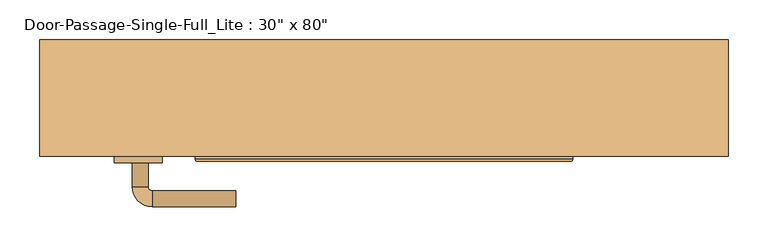
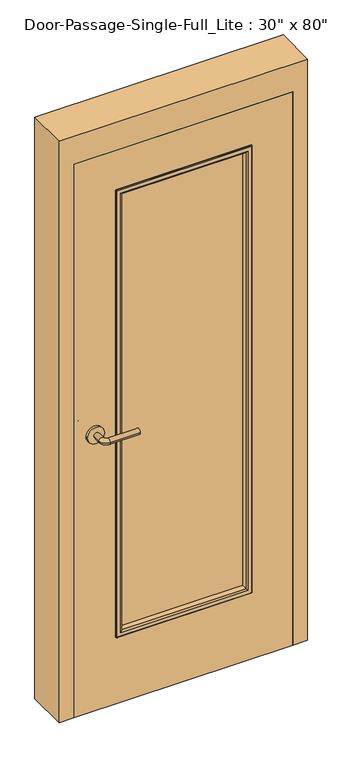
"""IFC4 building model written with IfcOpenShell, lengths in millimetres: door geometry."""

from ifc_helpers import new_model, si_unit, point, frame, frame_2d, origin, place, context, project, spatial, polyline, circle_curve, ellipse_curve, trimmed, segment, composite_curve, outline, extrude, faceted_brep, source, transform, mapped, element, save
from ifc_brep_helpers import plane_surface, cylinder_surface, revolved_surface, advanced_brep


def door_136239c3(model_context):
    return source(origin(), model_context, "Body", "SolidModel", [
        advanced_brep(
        [(-315.990625, -4.7, 1016.0), (-295.990625, -4.7, 1016.0), (-315.990625, 25.3, 1016.0), (-295.990625, 25.3, 1016.0), (-290.990625, 30.3, 1016.0), (-290.990625, 50.3, 1016.0), (-185.990625, 50.3, 1016.0), (-185.990625, 30.3, 1016.0)],
        [
            (0, 1, circle_curve(frame((-305.990625, -4.7, 1016.0), z_axis=(0.0, -1.0, 0.0), x_axis=(1.0, 0.0, 0.0)), 10.0)),
            (1, 0, circle_curve(frame((-305.990625, -4.7, 1016.0), z_axis=(0.0, -1.0, 0.0), x_axis=(1.0, 0.0, 0.0)), 10.0)),
            (0, 2),
            (2, 3, circle_curve(frame((-305.990625, 25.3, 1016.0), z_axis=(0.0, -1.0, 0.0), x_axis=(1.0, 0.0, 0.0)), 10.0)),
            (3, 1),
            (3, 2, circle_curve(frame((-305.990625, 25.3, 1016.0), z_axis=(0.0, -1.0, 0.0), x_axis=(1.0, 0.0, 0.0)), 10.0)),
            (4, 3, circle_curve(frame((-290.990625, 25.3, 1016.0), z_axis=(0.0, 0.0, 1.0), x_axis=(-1.0, 0.0, 0.0)), 5.0)),
            (2, 5, circle_curve(frame((-290.990625, 25.3, 1016.0), z_axis=(0.0, 0.0, -1.0), x_axis=(-1.0, 0.0, 0.0)), 25.0)),
            (5, 4, circle_curve(frame((-290.990625, 40.3, 1016.0), z_axis=(-1.0, 0.0, 0.0), x_axis=(0.0, -1.0, 0.0)), 10.0)),
            (4, 5, circle_curve(frame((-290.990625, 40.3, 1016.0), z_axis=(-1.0, 0.0, 0.0), x_axis=(0.0, -1.0, 0.0)), 10.0)),
            (6, 7, circle_curve(frame((-185.990625, 40.3, 1016.0), z_axis=(1.0, 0.0, 0.0), x_axis=(0.0, -1.0, 0.0)), 10.0)),
            (7, 6, circle_curve(frame((-185.990625, 40.3, 1016.0), z_axis=(1.0, 0.0, 0.0), x_axis=(0.0, -1.0, 0.0)), 10.0)),
            (5, 6),
            (7, 4),
        ],
        [
            plane_surface(frame((-305.990625, -4.7, 1016.0), z_axis=(0.0, -1.0, 0.0), x_axis=(0.0, 0.0, 1.0))),
            cylinder_surface(frame((-305.990625, -4.7, 1016.0), z_axis=(0.0, -1.0, 0.0), x_axis=(1.0, 0.0, 0.0)), 10.0),
            revolved_surface(trimmed(ellipse_curve(frame((-305.990625, 25.3, 1016.0), z_axis=(0.0, -1.0, 0.0), x_axis=(1.0, 0.0, 0.0)), 10.0, 10.0), [point((-315.990625, 25.3, 1016.0))], [point((-295.990625, 25.3, 1016.0))], True, "CARTESIAN"), (-290.990625, 25.3, 1016.0), (0.0, 0.0, -1.0)),
            revolved_surface(trimmed(ellipse_curve(frame((-305.990625, 25.3, 1016.0), z_axis=(0.0, -1.0, 0.0), x_axis=(1.0, 0.0, 0.0)), 10.0, 10.0), [point((-295.990625, 25.3, 1016.0))], [point((-315.990625, 25.3, 1016.0))], True, "CARTESIAN"), (-290.990625, 25.3, 1016.0), (0.0, 0.0, -1.0)),
            plane_surface(frame((-185.990625, 40.3, 1016.0), z_axis=(1.0, 0.0, 0.0), x_axis=(0.0, 0.0, 1.0))),
            cylinder_surface(frame((-290.990625, 40.3, 1016.0), z_axis=(-1.0, 0.0, 0.0), x_axis=(0.0, -1.0, 0.0)), 10.0),
        ],
        [
            (0, [[1, 2]]),
            (1, [[-1, 3, 4, 5]]),
            (1, [[-2, -5, 6, -3]]),
            (2, [[7, -4, 8, 9]]),
            (3, [[-8, -6, -7, 10]]),
            (4, [[11, 12]]),
            (5, [[-9, 13, -12, 14]]),
            (5, [[-10, -14, -11, -13]]),
        ],
    ),
        extrude(outline(composite_curve([segment(trimmed(circle_curve(frame_2d((1016.0, -308.490625)), 30.0), [point((1016.0, -338.490625))], [point((1016.0, -278.490625))], False, "CARTESIAN"), True, "CONTINUOUS"), segment(trimmed(circle_curve(frame_2d((1016.0, -308.490625)), 30.0), [point((1016.0, -278.490625))], [point((1016.0, -338.490625))], False, "CARTESIAN"), True, "CONTINUOUS")], self_intersect=False)), frame((0.0, -12.7, 0.0), z_axis=(0.0, 1.0, 0.0), x_axis=(0.0, 0.0, 1.0)), (0.0, 0.0, 1.0), 8.0),
        advanced_brep(
        [(-315.990625, -65.15, 1016.0), (-295.990625, -65.15, 1016.0), (-295.990625, -95.15, 1016.0), (-315.990625, -95.15, 1016.0), (-290.990625, -100.15, 1016.0), (-290.990625, -120.15, 1016.0), (-185.990625, -120.15, 1016.0), (-185.990625, -100.15, 1016.0)],
        [
            (0, 1, circle_curve(frame((-305.990625, -65.15, 1016.0), z_axis=(0.0, 1.0, 0.0), x_axis=(1.0, 0.0, 0.0)), 10.0)),
            (1, 0, circle_curve(frame((-305.990625, -65.15, 1016.0), z_axis=(0.0, 1.0, 0.0), x_axis=(1.0, 0.0, 0.0)), 10.0)),
            (1, 2),
            (2, 3, circle_curve(frame((-305.990625, -95.15, 1016.0), z_axis=(0.0, 1.0, 0.0), x_axis=(1.0, 0.0, 0.0)), 10.0)),
            (3, 0),
            (3, 2, circle_curve(frame((-305.990625, -95.15, 1016.0), z_axis=(0.0, 1.0, 0.0), x_axis=(1.0, 0.0, 0.0)), 10.0)),
            (4, 5, circle_curve(frame((-290.990625, -110.15, 1016.0), z_axis=(-1.0, 0.0, 0.0), x_axis=(0.0, 1.0, 0.0)), 10.0)),
            (5, 3, circle_curve(frame((-290.990625, -95.15, 1016.0), z_axis=(0.0, 0.0, -1.0), x_axis=(-1.0, 0.0, 0.0)), 25.0)),
            (2, 4, circle_curve(frame((-290.990625, -95.15, 1016.0), z_axis=(0.0, 0.0, 1.0), x_axis=(-1.0, 0.0, 0.0)), 5.0)),
            (5, 4, circle_curve(frame((-290.990625, -110.15, 1016.0), z_axis=(-1.0, 0.0, 0.0), x_axis=(0.0, 1.0, 0.0)), 10.0)),
            (6, 7, circle_curve(frame((-185.990625, -110.15, 1016.0), z_axis=(1.0, 0.0, 0.0), x_axis=(0.0, 1.0, 0.0)), 10.0)),
            (7, 6, circle_curve(frame((-185.990625, -110.15, 1016.0), z_axis=(1.0, 0.0, 0.0), x_axis=(0.0, 1.0, 0.0)), 10.0)),
            (4, 7),
            (6, 5),
        ],
        [
            plane_surface(frame((-305.990625, -65.15, 1016.0), z_axis=(0.0, 1.0, 0.0), x_axis=(0.0, 0.0, 1.0))),
            cylinder_surface(frame((-305.990625, -65.15, 1016.0), z_axis=(0.0, 1.0, 0.0), x_axis=(1.0, 0.0, 0.0)), 10.0),
            revolved_surface(trimmed(ellipse_curve(frame((-305.990625, -95.15, 1016.0), z_axis=(0.0, -1.0, 0.0), x_axis=(1.0, 0.0, 0.0)), 10.0, 10.0), [point((-315.990625, -95.15, 1016.0))], [point((-295.990625, -95.15, 1016.0))], True, "CARTESIAN"), (-290.990625, -95.15, 1016.0), (0.0, 0.0, -1.0)),
            revolved_surface(trimmed(ellipse_curve(frame((-305.990625, -95.15, 1016.0), z_axis=(0.0, -1.0, 0.0), x_axis=(1.0, 0.0, 0.0)), 10.0, 10.0), [point((-295.990625, -95.15, 1016.0))], [point((-315.990625, -95.15, 1016.0))], True, "CARTESIAN"), (-290.990625, -95.15, 1016.0), (0.0, 0.0, -1.0)),
            plane_surface(frame((-185.990625, -110.15, 1016.0), z_axis=(1.0, 0.0, 0.0), x_axis=(0.0, 0.0, 1.0))),
            cylinder_surface(frame((-290.990625, -110.15, 1016.0), z_axis=(-1.0, 0.0, 0.0), x_axis=(0.0, 1.0, 0.0)), 10.0),
        ],
        [
            (0, [[1, 2]]),
            (1, [[3, 4, 5, -2]]),
            (1, [[-5, 6, -3, -1]]),
            (2, [[7, 8, -4, 9]]),
            (3, [[10, -9, -6, -8]]),
            (4, [[11, 12]]),
            (5, [[13, -11, 14, -7]]),
            (5, [[-14, -12, -13, -10]]),
        ],
    ),
        extrude(outline(composite_curve([segment(trimmed(circle_curve(frame_2d((1016.0, -308.490625)), 30.0), [point((1016.0, -338.490625))], [point((1016.0, -278.490625))], False, "CARTESIAN"), True, "CONTINUOUS"), segment(trimmed(circle_curve(frame_2d((1016.0, -308.490625)), 30.0), [point((1016.0, -278.490625))], [point((1016.0, -338.490625))], False, "CARTESIAN"), True, "CONTINUOUS")], self_intersect=False)), frame((0.0, -65.15, 0.0), z_axis=(0.0, 1.0, 0.0), x_axis=(0.0, 0.0, 1.0)), (0.0, 0.0, 1.0), 8.0),
        extrude(outline(polyline([(228.6, -31.75), (228.6, -38.1), (-228.6, -38.1), (-228.6, -31.75), (228.6, -31.75)])), frame((0.0, 0.0, 254.0), z_axis=(0.0, 0.0, 1.0), x_axis=(1.0, 0.0, 0.0)), (0.0, 0.0, 1.0), 1625.6),
        faceted_brep([(381.0, -7.9375, 0.0), (365.125, -7.9375, 0.0), (365.125, 39.6875, 0.0), (381.0, 39.6875, 0.0), (381.0, 88.9, 0.0), (431.8, 88.9, 0.0), (431.8, -57.15, 0.0), (381.0, -57.15, 0.0), (381.0, -57.15, 2032.0), (381.0, -7.9375, 2032.0), (431.8, -57.15, 2133.6), (-431.8, -57.15, 2133.6), (-431.8, -57.15, 0.0), (-381.0, -57.15, 0.0), (-381.0, -57.15, 2032.0), (431.8, 88.9, 2133.6), (381.0, 88.9, 2032.0), (-381.0, 88.9, 2032.0), (-381.0, 88.9, 0.0), (-431.8, 88.9, 0.0), (-431.8, 88.9, 2133.6), (381.0, 39.6875, 2032.0), (365.125, 39.6875, 2016.125), (-365.125, 39.6875, 2016.125), (-365.125, 39.6875, 0.0), (-381.0, 39.6875, 0.0), (-381.0, 39.6875, 2032.0), (365.125, -7.9375, 2016.125), (-381.0, -7.9375, 2032.0), (-381.0, -7.9375, 0.0), (-365.125, -7.9375, 0.0), (-365.125, -7.9375, 2016.125)], [[[0, 1, 2, 3, 4, 5, 6, 7]], [[7, 8, 9, 0]], [[6, 10, 11, 12, 13, 14, 8, 7]], [[5, 15, 10, 6]], [[4, 16, 17, 18, 19, 20, 15, 5]], [[3, 21, 16, 4]], [[2, 22, 23, 24, 25, 26, 21, 3]], [[1, 27, 22, 2]], [[0, 9, 28, 29, 30, 31, 27, 1]], [[8, 14, 28, 9]], [[16, 21, 26, 17]], [[22, 27, 31, 23]], [[12, 19, 18, 25, 24, 30, 29, 13]], [[13, 29, 28, 14]], [[11, 20, 19, 12]], [[17, 26, 25, 18]], [[23, 31, 30, 24]], [[15, 20, 11, 10]]]),
        extrude(outline(polyline([(2032.0, -381.0), (0.0, -381.0), (0.0, 381.0), (2032.0, 381.0), (2032.0, -381.0)]), holes=[polyline([(1879.6, -228.6), (1879.6, 228.6), (254.0, 228.6), (254.0, -228.6), (1879.6, -228.6)])]), frame((0.0, -57.15, 0.0), z_axis=(0.0, 1.0, 0.0), x_axis=(0.0, 0.0, 1.0)), (0.0, 0.0, 1.0), 44.45),
        advanced_brep(
        [(-228.6, -38.1, 1879.6), (-228.6, -38.1, 254.0), (-228.6, -57.15, 254.0), (-228.6, -57.15, 1879.6), (-216.6, -58.15, 1867.6), (-216.6, -58.15, 266.0), (-216.6, -38.1, 266.0), (-216.6, -38.1, 1867.6), (-221.6, -63.15, 1872.6), (-221.6, -63.15, 261.0), (-236.6, -61.15, 1887.6), (-236.6, -61.15, 246.0), (-234.6, -63.15, 248.0), (-234.6, -63.15, 1885.6), (-236.6, -57.15, 1887.6), (-236.6, -57.15, 246.0), (228.6, -38.1, 254.0), (228.6, -57.15, 254.0), (216.6, -58.15, 266.0), (216.6, -38.1, 266.0), (221.6, -63.15, 261.0), (236.6, -61.15, 246.0), (234.6, -63.15, 248.0), (236.6, -57.15, 246.0), (228.6, -38.1, 1879.6), (228.6, -57.15, 1879.6), (216.6, -58.15, 1867.6), (216.6, -38.1, 1867.6), (221.6, -63.15, 1872.6), (236.6, -61.15, 1887.6), (234.6, -63.15, 1885.6), (236.6, -57.15, 1887.6)],
        [
            (0, 1),
            (1, 2),
            (2, 3),
            (3, 0),
            (4, 5),
            (5, 6),
            (6, 7),
            (7, 4),
            (8, 9),
            (9, 5, ellipse_curve(frame((-221.6, -58.15, 261.0), z_axis=(-0.7071067811865475, 0.0, 0.7071067811865475), x_axis=(0.7071067811865474, 0.0, 0.7071067811865476)), 7.0710678, 5.0)),
            (4, 8, ellipse_curve(frame((-221.6, -58.15, 1872.6), z_axis=(-0.7071067811865475, 0.0, -0.7071067811865475), x_axis=(-0.7071067811865474, 0.0, 0.7071067811865476)), 7.0710678, 5.0)),
            (10, 11),
            (11, 12, ellipse_curve(frame((-234.6, -61.15, 248.0), z_axis=(-0.7071067811865475, 0.0, 0.7071067811865475), x_axis=(0.7071067811865474, 0.0, 0.7071067811865476)), 2.8284271, 2.0)),
            (12, 13),
            (13, 10, ellipse_curve(frame((-234.6, -61.15, 1885.6), z_axis=(-0.7071067811865475, 0.0, -0.7071067811865475), x_axis=(-0.7071067811865474, 0.0, 0.7071067811865476)), 2.8284271, 2.0)),
            (14, 15),
            (15, 11),
            (10, 14),
            (1, 16),
            (16, 17),
            (17, 2),
            (5, 18),
            (18, 19),
            (19, 6),
            (9, 20),
            (20, 18, ellipse_curve(frame((221.6, -58.15, 261.0), z_axis=(-0.7071067811865475, 0.0, -0.7071067811865475), x_axis=(-0.7071067811865476, 0.0, 0.7071067811865474)), 7.0710678, 5.0)),
            (11, 21),
            (21, 22, ellipse_curve(frame((234.6, -61.15, 248.0), z_axis=(-0.7071067811865475, 0.0, -0.7071067811865475), x_axis=(-0.7071067811865476, 0.0, 0.7071067811865474)), 2.8284271, 2.0)),
            (22, 12),
            (15, 23),
            (23, 21),
            (16, 24),
            (24, 25),
            (25, 17),
            (18, 26),
            (26, 27),
            (27, 19),
            (20, 28),
            (28, 26, ellipse_curve(frame((221.6, -58.15, 1872.6), z_axis=(0.7071067811865475, 0.0, -0.7071067811865475), x_axis=(-0.7071067811865474, 0.0, -0.7071067811865476)), 7.0710678, 5.0)),
            (21, 29),
            (29, 30, ellipse_curve(frame((234.6, -61.15, 1885.6), z_axis=(0.7071067811865475, 0.0, -0.7071067811865475), x_axis=(-0.7071067811865474, 0.0, -0.7071067811865476)), 2.8284271, 2.0)),
            (30, 22),
            (23, 31),
            (31, 29),
            (14, 31),
            (25, 3),
            (24, 0),
            (27, 7),
            (26, 4),
            (28, 8),
            (30, 13),
            (29, 10),
        ],
        [
            plane_surface(frame((-228.6, -57.15, 1879.6), z_axis=(-1.0, 0.0, 0.0), x_axis=(0.0, 0.0, -1.0))),
            plane_surface(frame((-216.6, -38.1, 1867.6), z_axis=(1.0, 0.0, 0.0), x_axis=(0.0, 0.0, -1.0))),
            cylinder_surface(frame((-221.6, -58.15, 1879.6), z_axis=(0.0, 0.0, 1.0), x_axis=(-1.0, 0.0, 0.0)), 5.0),
            cylinder_surface(frame((-234.6, -61.15, 1879.6), z_axis=(0.0, 0.0, 1.0), x_axis=(-1.0, 0.0, 0.0)), 2.0),
            plane_surface(frame((-236.6, -61.15, 1887.6), z_axis=(-1.0, 0.0, 0.0), x_axis=(0.0, 0.0, -1.0))),
            plane_surface(frame((-228.6, -57.15, 254.0), z_axis=(0.0, 0.0, -1.0), x_axis=(1.0, 0.0, 0.0))),
            plane_surface(frame((-216.6, -38.1, 266.0), z_axis=(0.0, 0.0, 1.0), x_axis=(1.0, 0.0, 0.0))),
            cylinder_surface(frame((-228.6, -58.15, 261.0), z_axis=(-1.0, 0.0, 0.0), x_axis=(0.0, 0.0, -1.0)), 5.0),
            cylinder_surface(frame((-228.6, -61.15, 248.0), z_axis=(-1.0, 0.0, 0.0), x_axis=(0.0, 0.0, -1.0)), 2.0),
            plane_surface(frame((-236.6, -61.15, 246.0), z_axis=(0.0, 0.0, -1.0), x_axis=(1.0, 0.0, 0.0))),
            plane_surface(frame((228.6, -57.15, 254.0), z_axis=(1.0, 0.0, 0.0), x_axis=(0.0, 0.0, 1.0))),
            plane_surface(frame((216.6, -38.1, 266.0), z_axis=(-1.0, 0.0, 0.0), x_axis=(0.0, 0.0, 1.0))),
            cylinder_surface(frame((221.6, -58.15, 254.0), z_axis=(0.0, 0.0, -1.0), x_axis=(1.0, 0.0, 0.0)), 5.0),
            cylinder_surface(frame((234.6, -61.15, 254.0), z_axis=(0.0, 0.0, -1.0), x_axis=(1.0, 0.0, 0.0)), 2.0),
            plane_surface(frame((236.6, -61.15, 246.0), z_axis=(1.0, 0.0, 0.0), x_axis=(0.0, 0.0, 1.0))),
            plane_surface(frame((236.6, -57.15, 1887.6), z_axis=(0.0, 1.0, 0.0), x_axis=(-1.0, 0.0, 0.0))),
            plane_surface(frame((228.6, -57.15, 1879.6), z_axis=(0.0, 0.0, 1.0), x_axis=(-1.0, 0.0, 0.0))),
            plane_surface(frame((228.6, -38.1, 1879.6), z_axis=(0.0, 1.0, 0.0), x_axis=(-1.0, 0.0, 0.0))),
            plane_surface(frame((216.6, -38.1, 1867.6), z_axis=(0.0, 0.0, -1.0), x_axis=(-1.0, 0.0, 0.0))),
            cylinder_surface(frame((228.6, -58.15, 1872.6), z_axis=(1.0, 0.0, 0.0), x_axis=(0.0, 0.0, 1.0)), 5.0),
            plane_surface(frame((221.6, -63.15, 1872.6), z_axis=(0.0, -1.0, 0.0), x_axis=(-1.0, 0.0, 0.0))),
            cylinder_surface(frame((228.6, -61.15, 1885.6), z_axis=(1.0, 0.0, 0.0), x_axis=(0.0, 0.0, 1.0)), 2.0),
            plane_surface(frame((236.6, -61.15, 1887.6), z_axis=(0.0, 0.0, 1.0), x_axis=(-1.0, 0.0, 0.0))),
        ],
        [
            (0, [[1, 2, 3, 4]]),
            (1, [[5, 6, 7, 8]]),
            (2, [[9, 10, -5, 11]]),
            (3, [[12, 13, 14, 15]]),
            (4, [[16, 17, -12, 18]]),
            (5, [[19, 20, 21, -2]]),
            (6, [[22, 23, 24, -6]]),
            (7, [[25, 26, -22, -10]]),
            (8, [[27, 28, 29, -13]]),
            (9, [[30, 31, -27, -17]]),
            (10, [[32, 33, 34, -20]]),
            (11, [[35, 36, 37, -23]]),
            (12, [[38, 39, -35, -26]]),
            (13, [[40, 41, 42, -28]]),
            (14, [[43, 44, -40, -31]]),
            (15, [[-16, 45, -43, -30], [-3, -21, -34, 46]]),
            (16, [[47, -4, -46, -33]]),
            (17, [[-1, -47, -32, -19], [-7, -24, -37, 48]]),
            (18, [[49, -8, -48, -36]]),
            (19, [[50, -11, -49, -39]]),
            (20, [[-14, -29, -42, 51], [-9, -50, -38, -25]]),
            (21, [[52, -15, -51, -41]]),
            (22, [[-45, -18, -52, -44]]),
        ],
    ),
        advanced_brep(
        [(-228.6, -31.75, 254.0), (-228.6, -31.75, 1879.6), (-228.6, -12.7, 1879.6), (-228.6, -12.7, 254.0), (-216.6, -11.7, 266.0), (-216.6, -11.7, 1867.6), (-216.6, -31.75, 1867.6), (-216.6, -31.75, 266.0), (-221.6, -6.7, 261.0), (-221.6, -6.7, 1872.6), (-236.6, -8.7, 246.0), (-236.6, -8.7, 1887.6), (-234.6, -6.7, 1885.6), (-234.6, -6.7, 248.0), (-236.6, -12.7, 246.0), (-236.6, -12.7, 1887.6), (228.6, -31.75, 1879.6), (228.6, -12.7, 1879.6), (216.6, -11.7, 1867.6), (216.6, -31.75, 1867.6), (221.6, -6.7, 1872.6), (236.6, -8.7, 1887.6), (234.6, -6.7, 1885.6), (236.6, -12.7, 1887.6), (228.6, -31.75, 254.0), (228.6, -12.7, 254.0), (216.6, -11.7, 266.0), (216.6, -31.75, 266.0), (221.6, -6.7, 261.0), (236.6, -8.7, 246.0), (234.6, -6.7, 248.0), (236.6, -12.7, 246.0)],
        [
            (0, 1),
            (1, 2),
            (2, 3),
            (3, 0),
            (4, 5),
            (5, 6),
            (6, 7),
            (7, 4),
            (8, 9),
            (9, 5, ellipse_curve(frame((-221.6, -11.7, 1872.6), z_axis=(-0.7071067811865475, 0.0, -0.7071067811865475), x_axis=(0.7071067811865474, 0.0, -0.7071067811865476)), 7.0710678, 5.0)),
            (4, 8, ellipse_curve(frame((-221.6, -11.7, 261.0), z_axis=(-0.7071067811865475, 0.0, 0.7071067811865475), x_axis=(-0.7071067811865474, 0.0, -0.7071067811865476)), 7.0710678, 5.0)),
            (10, 11),
            (11, 12, ellipse_curve(frame((-234.6, -8.7, 1885.6), z_axis=(-0.7071067811865475, 0.0, -0.7071067811865475), x_axis=(0.7071067811865474, 0.0, -0.7071067811865476)), 2.8284271, 2.0)),
            (12, 13),
            (13, 10, ellipse_curve(frame((-234.6, -8.7, 248.0), z_axis=(-0.7071067811865475, 0.0, 0.7071067811865475), x_axis=(-0.7071067811865474, 0.0, -0.7071067811865476)), 2.8284271, 2.0)),
            (14, 15),
            (15, 11),
            (10, 14),
            (1, 16),
            (16, 17),
            (17, 2),
            (5, 18),
            (18, 19),
            (19, 6),
            (9, 20),
            (20, 18, ellipse_curve(frame((221.6, -11.7, 1872.6), z_axis=(-0.7071067811865475, 0.0, 0.7071067811865475), x_axis=(-0.7071067811865476, 0.0, -0.7071067811865474)), 7.0710678, 5.0)),
            (11, 21),
            (21, 22, ellipse_curve(frame((234.6, -8.7, 1885.6), z_axis=(-0.7071067811865475, 0.0, 0.7071067811865475), x_axis=(-0.7071067811865476, 0.0, -0.7071067811865474)), 2.8284271, 2.0)),
            (22, 12),
            (15, 23),
            (23, 21),
            (16, 24),
            (24, 25),
            (25, 17),
            (18, 26),
            (26, 27),
            (27, 19),
            (20, 28),
            (28, 26, ellipse_curve(frame((221.6, -11.7, 261.0), z_axis=(0.7071067811865475, 0.0, 0.7071067811865475), x_axis=(-0.7071067811865474, 0.0, 0.7071067811865476)), 7.0710678, 5.0)),
            (21, 29),
            (29, 30, ellipse_curve(frame((234.6, -8.7, 248.0), z_axis=(0.7071067811865475, 0.0, 0.7071067811865475), x_axis=(-0.7071067811865474, 0.0, 0.7071067811865476)), 2.8284271, 2.0)),
            (30, 22),
            (23, 31),
            (31, 29),
            (14, 31),
            (25, 3),
            (24, 0),
            (27, 7),
            (26, 4),
            (28, 8),
            (30, 13),
            (29, 10),
        ],
        [
            plane_surface(frame((-228.6, -12.7, 254.0), z_axis=(-1.0, 0.0, 0.0), x_axis=(0.0, 0.0, 1.0))),
            plane_surface(frame((-216.6, -31.75, 266.0), z_axis=(1.0, 0.0, 0.0), x_axis=(0.0, 0.0, 1.0))),
            cylinder_surface(frame((-221.6, -11.7, 254.0), z_axis=(0.0, 0.0, -1.0), x_axis=(-1.0, 0.0, 0.0)), 5.0),
            cylinder_surface(frame((-234.6, -8.7, 254.0), z_axis=(0.0, 0.0, -1.0), x_axis=(-1.0, 0.0, 0.0)), 2.0),
            plane_surface(frame((-236.6, -8.7, 246.0), z_axis=(-1.0, 0.0, 0.0), x_axis=(0.0, 0.0, 1.0))),
            plane_surface(frame((-228.6, -12.7, 1879.6), z_axis=(0.0, 0.0, 1.0), x_axis=(1.0, 0.0, 0.0))),
            plane_surface(frame((-216.6, -31.75, 1867.6), z_axis=(0.0, 0.0, -1.0), x_axis=(1.0, 0.0, 0.0))),
            cylinder_surface(frame((-228.6, -11.7, 1872.6), z_axis=(-1.0, 0.0, 0.0), x_axis=(0.0, 0.0, 1.0)), 5.0),
            cylinder_surface(frame((-228.6, -8.7, 1885.6), z_axis=(-1.0, 0.0, 0.0), x_axis=(0.0, 0.0, 1.0)), 2.0),
            plane_surface(frame((-236.6, -8.7, 1887.6), z_axis=(0.0, 0.0, 1.0), x_axis=(1.0, 0.0, 0.0))),
            plane_surface(frame((228.6, -12.7, 1879.6), z_axis=(1.0, 0.0, 0.0), x_axis=(0.0, 0.0, -1.0))),
            plane_surface(frame((216.6, -31.75, 1867.6), z_axis=(-1.0, 0.0, 0.0), x_axis=(0.0, 0.0, -1.0))),
            cylinder_surface(frame((221.6, -11.7, 1879.6), z_axis=(0.0, 0.0, 1.0), x_axis=(1.0, 0.0, 0.0)), 5.0),
            cylinder_surface(frame((234.6, -8.7, 1879.6), z_axis=(0.0, 0.0, 1.0), x_axis=(1.0, 0.0, 0.0)), 2.0),
            plane_surface(frame((236.6, -8.7, 1887.6), z_axis=(1.0, 0.0, 0.0), x_axis=(0.0, 0.0, -1.0))),
            plane_surface(frame((236.6, -12.7, 246.0), z_axis=(0.0, -1.0, 0.0), x_axis=(-1.0, 0.0, 0.0))),
            plane_surface(frame((228.6, -12.7, 254.0), z_axis=(0.0, 0.0, -1.0), x_axis=(-1.0, 0.0, 0.0))),
            plane_surface(frame((228.6, -31.75, 254.0), z_axis=(0.0, -1.0, 0.0), x_axis=(-1.0, 0.0, 0.0))),
            plane_surface(frame((216.6, -31.75, 266.0), z_axis=(0.0, 0.0, 1.0), x_axis=(-1.0, 0.0, 0.0))),
            cylinder_surface(frame((228.6, -11.7, 261.0), z_axis=(1.0, 0.0, 0.0), x_axis=(0.0, 0.0, -1.0)), 5.0),
            plane_surface(frame((221.6, -6.7, 261.0), z_axis=(0.0, 1.0, 0.0), x_axis=(-1.0, 0.0, 0.0))),
            cylinder_surface(frame((228.6, -8.7, 248.0), z_axis=(1.0, 0.0, 0.0), x_axis=(0.0, 0.0, -1.0)), 2.0),
            plane_surface(frame((236.6, -8.7, 246.0), z_axis=(0.0, 0.0, -1.0), x_axis=(-1.0, 0.0, 0.0))),
        ],
        [
            (0, [[1, 2, 3, 4]]),
            (1, [[5, 6, 7, 8]]),
            (2, [[9, 10, -5, 11]]),
            (3, [[12, 13, 14, 15]]),
            (4, [[16, 17, -12, 18]]),
            (5, [[19, 20, 21, -2]]),
            (6, [[22, 23, 24, -6]]),
            (7, [[25, 26, -22, -10]]),
            (8, [[27, 28, 29, -13]]),
            (9, [[30, 31, -27, -17]]),
            (10, [[32, 33, 34, -20]]),
            (11, [[35, 36, 37, -23]]),
            (12, [[38, 39, -35, -26]]),
            (13, [[40, 41, 42, -28]]),
            (14, [[43, 44, -40, -31]]),
            (15, [[-16, 45, -43, -30], [-3, -21, -34, 46]]),
            (16, [[47, -4, -46, -33]]),
            (17, [[-1, -47, -32, -19], [-7, -24, -37, 48]]),
            (18, [[49, -8, -48, -36]]),
            (19, [[50, -11, -49, -39]]),
            (20, [[-14, -29, -42, 51], [-9, -50, -38, -25]]),
            (21, [[52, -15, -51, -41]]),
            (22, [[-45, -18, -52, -44]]),
        ],
    ),
    ])


if __name__ == "__main__":
    model = new_model("IFC4")
    model_context = context("Model", 3, world=origin())
    ifc_project = project(units=[si_unit("LENGTHUNIT", "METRE", prefix="MILLI")], contexts=[model_context])
    site = spatial("IfcSite", under=ifc_project)
    building = spatial("IfcBuilding", under=site)
    placement = place(None, origin())
    door_shape = door_136239c3(model_context)
    element("IfcDoor", 1, ObjectType="Door-Passage-Single-Full_Lite : 30\" x 80\"", at=placement, inside=building, context=model_context, shape_type="MappedRepresentation", body=[
        mapped(door_shape, transform((0.0, 0.0, 0.0), x_axis=(1.0, 0.0, 0.0), y_axis=(0.0, 1.0, 0.0), z_axis=(0.0, 0.0, 1.0))),
    ])
    save(model, "model.ifc")

# Revit data of these elements
# Type "Door-Passage-Single-Full_Lite : 30\" x 80\""
#   Type Mark = "13"
#   Assembly Code = "B2030100"
#   Analytic Construction = "Wooden"
#   Thickness = 0' - 1 3/4"
#   Thermal Resistance (R) = 2.5876 (h·ft²·°F)/BTU
#   Swing Angle [instance default] = 90.00°
#   Strike Height = 3' - 4"
#   Rough Width [instance default] = 2' - 10"
#   Rough Height [instance default] = 7' - 0"
#   MF Opening Height [instance default] = 0' - 4"
#   MF Opening Width [instance default] = 0' - 4"
#   Inset Calculate [instance default] = 0' - 4"
#   Masonry Inset [instance default] = 0' - 1"
#   Height = 6' - 8"
#   Width = 2' - 6"
#   Heat Transfer Coefficient (U) = 0.3865 BTU/(h·ft²·°F)
#   Masonry Frame Depth = 0' - 5 3/4"
#   Masonry Frame [instance default] = yes
#   Function = 1
#   Dry Wall Frame [instance default] = no
#   Panel Material = Wood - Birch
#   Glazing = Glass
#   Glass Stop Material = Metal - Paint Finish - Grey
#   Frame Material = Metal - Paint Finish - Grey
#   Door Handle Material = Aluminum
#   Visual Light Transmittance = 0
#   Solar Heat Gain Coefficient = 0
#   Wall Closure = (empty or 0)
# Element 1 (IfcDoor, "Door-Passage-Single-Full_Lite : 30\" x 80\"")
#   Materials on its faces: "Metal - Paint Finish - Grey", "Aluminum", "Wood - Birch", "Glass"
# Materials
#   "Wood - Birch": class "Wood", colour RGB 166 116 52, transparency 0, Cost = 0
#   "Glass": class "Glass", colour RGB 0 128 192, transparency 0.75, Description = "Soda Lime Glass", Cost = 0
#   "Metal - Paint Finish - Grey": class "Paint", colour RGB 104 104 104, transparency 0, Cost = 0
#   "Aluminum": class "Metal", colour RGB 247 247 247, transparency 0, Description = "Aluminum 6061", Cost = 0
